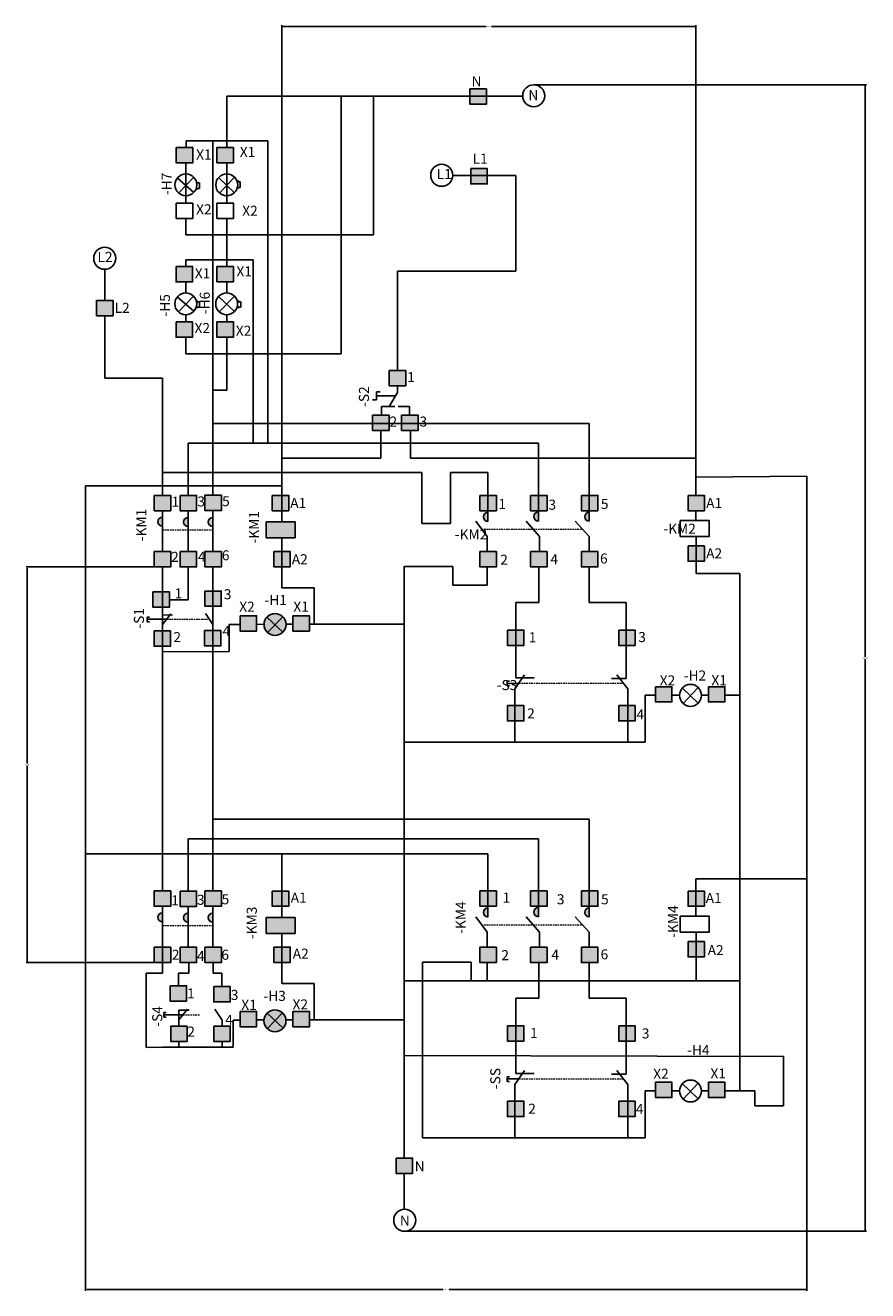
# Model space of a CAD drawing. Units: inches. Extents: x 892 to 1021, y 674 to 867.
import ezdxf

# ---------------------------------------------------------------- set-up
doc = ezdxf.new("R2010")
doc.units = ezdxf.units.IN
doc.header["$MEASUREMENT"] = 0
doc.linetypes.add('DASHED2', pattern=[0.375, 0.25, -0.125])
for name, color, linetype, lineweight in [('A-ANNO-DIMS', 2, 'Continuous', 18), ('E-ANNO-TAGS', 4, 'Continuous', 18), ('E-ANNO-TEXT', 4, 'Continuous', 18), ('E-CTRL-COIL', 7, 'Continuous', 25), ('E-CTRL-CONT', 7, 'Continuous', 25), ('E-CTRL-LAMP', 7, 'Continuous', 25), ('E-CTRL-LINK', 7, 'DASHED2', 18), ('E-CTRL-SWCH', 7, 'Continuous', 25), ('E-CTRL-TERM', 7, 'Continuous', 25), ('E-CTRL-WIRE', 7, 'Continuous', 25), ('E-LAMP-PATT', 1, 'Continuous', 13), ('E-POWR-PORT', 7, 'Continuous', 25), ('E-SYMB-PATT', 7, 'Continuous', 13), ('E-WIRE-NEUT', 4, 'Continuous', 25)]:
    doc.layers.add(name, color=color, linetype=linetype, lineweight=lineweight)
for name, color, linetype, lineweight, true_color in [('E-COIL-PATT', 2, 'Continuous', 13, 0xf1eb1f), ('E-WIRE-L1', 30, 'Continuous', 25, 0xf26722), ('E-WIRE-L2', 219, 'Continuous', 25, 0x642165)]:
    doc.layers.add(name, color=color, linetype=linetype, lineweight=lineweight, true_color=true_color)
doc.styles.get("Standard").update_dxf_attribs({"font": 'arial.ttf'})
doc.dimstyles.get("Standard").update_dxf_attribs({"dimtxt": 0.18, "dimasz": 0.18, "dimexe": 0.18, "dimexo": 0.0625, "dimgap": 0.09, "dimtad": 0, "dimtih": 1, "dimtoh": 1, "dimdec": 4, "dimzin": 0, "dimdsep": 46, "dimtxsty": 'Standard', "dimcen": 0.09, "dimadec": 0, "dimazin": 0, "dimtfac": 1, "dimtdec": 4, "dimtofl": 0, "dimtmove": 0, "dimatfit": 3, "dimfxl": 1, "dimtolj": 1, "dimtzin": 0, "dimarcsym": 0})

# ---------------------------------------------------------------- blocks, each defined once
blk = doc.blocks.new('KM-3POLE-CLOSED')
for p, q in [((1.25, 8.6), (1.25, 2.34)), ((5.18, 8.59), (5.18, 2.34)), ((8.95, 8.62), (8.95, 2.34))]:
    blk.add_line(p, q)
for points in [[(0, 10.95), (2.52, 10.95), (2.52, 8.6), (0, 8.6)], [(3.96, 10.93), (6.48, 10.93), (6.48, 8.59), (3.96, 8.59)], [(7.74, 10.96), (10.26, 10.96), (10.26, 8.62), (7.74, 8.62)], [(0, 2.34), (2.52, 2.34), (2.52, 0), (0, 0)], [(3.96, 2.34), (6.48, 2.34), (6.48, 0), (3.96, 0)], [(7.74, 2.34), (10.26, 2.34), (10.26, 0), (7.74, 0)]]:
    blk.add_lwpolyline(points, close=True)
for centre in [(1.25, 6.92), (5.18, 6.87), (8.95, 6.87)]:
    blk.add_arc(centre, 0.695, 90, 270)
blk = doc.blocks.new('KM-3POLE-OPEN')
for p, q in [((1.87, 10.95), (1.87, 6.96)), ((9.59, 10.95), (9.59, 7.01)), ((17.36, 10.95), (17.36, 6.98)), ((1.73, 4.63), (0, 7)), ((9.77, 4.63), (7.7, 7)), ((15.23, 7), (17.36, 4.63)), ((1.73, 2.34), (1.73, 4.63)), ((9.77, 2.34), (9.77, 4.63)), ((17.36, 4.63), (17.37, 2.34))]:
    blk.add_line(p, q)
for points in [[(0.65, 10.95), (3.17, 10.95), (3.17, 8.6), (0.65, 8.6)], [(8.39, 10.95), (10.91, 10.95), (10.91, 8.6), (8.39, 8.6)], [(16.16, 10.95), (18.68, 10.95), (18.68, 8.6), (16.16, 8.6)], [(0.65, 2.34), (3.17, 2.34), (3.17, 0), (0.65, 0)], [(8.39, 2.34), (10.91, 2.34), (10.91, 0), (8.39, 0)], [(16.16, 2.34), (18.68, 2.34), (18.68, 0), (16.16, 0)]]:
    blk.add_lwpolyline(points, close=True)
for centre in [(1.87, 7.66), (9.59, 7.71), (17.36, 7.67)]:
    blk.add_arc(centre, 0.695, 90, 270)
blk = doc.blocks.new('PB-LINKED-PAIR')
for p, q in [((1.31, 13.88), (1.31, 6.6)), ((18.2, 13.88), (18.21, 6.5)), ((0, 5.74), (0, 6.09)), ((0, 6.09), (0.36, 6.09)), ((1.14, 4.89), (2.64, 7.04)), ((1.31, 6.6), (4.09, 6.6)), ((18.21, 6.5), (15.96, 6.5)), ((18.45, 4.89), (16.77, 7.04)), ((1.73, 5.74), (0, 5.74)), ((0, 5.38), (0, 5.74)), ((0.36, 5.38), (0, 5.38)), ((1.14, 0), (1.14, 4.89)), ((18.45, 0), (18.45, 4.89))]:
    blk.add_line(p, q)
for points in [[(0.02, 13.88), (2.55, 13.88), (2.55, 11.54), (0.02, 11.54)], [(17.04, 13.88), (19.56, 13.88), (19.56, 11.54), (17.04, 11.54)], [(0.02, 2.34), (2.55, 2.34), (2.55, 0), (0.02, 0)], [(17.04, 2.34), (19.56, 2.34), (19.56, 0), (17.04, 0)]]:
    blk.add_lwpolyline(points, close=True)
blk = doc.blocks.new('KM-COIL')
for p, q in [((2.4, 7.73), (2.4, 6.11)), ((2.42, 3.79), (2.43, 2.34))]:
    blk.add_line(p, q)
for points in [[(1.19, 10.07), (3.71, 10.07), (3.71, 7.73), (1.19, 7.73)], [(0, 6.21), (4.44, 6.21), (4.44, 3.79), (0, 3.79)], [(1.19, 2.34), (3.71, 2.34), (3.71, 0), (1.19, 0)]]:
    blk.add_lwpolyline(points, close=True)
blk = doc.blocks.new('PILOT-LAMP-H')
for p, q in [((6.53, 0.48), (4.1, 2.81)), ((4.22, 0.43), (6.54, 2.87)), ((3.67, 1.71), (2.52, 1.7)), ((8.09, 1.72), (7.03, 1.73))]:
    blk.add_line(p, q)
for points in [[(0, 3.01), (2.52, 3.01), (2.52, 0.67), (0, 0.67)], [(8.09, 3.01), (10.61, 3.01), (10.61, 0.67), (8.09, 0.67)]]:
    blk.add_lwpolyline(points, close=True)
blk.add_circle((5.35, 1.68), 1.68)
blk = doc.blocks.new('PILOT-LAMP-V1')
for p, q in [((1.68, 8.48), (1.68, 6.8)), ((2.91, 3.97), (0.37, 6.17)), ((0.55, 3.87), (2.88, 6.3)), ((1.68, 5.05), (1.68, 5.03)), ((1.68, 3.44), (1.68, 2.34))]:
    blk.add_line(p, q)
for points in [[(0.21, 10.83), (2.73, 10.83), (2.73, 8.48), (0.21, 8.48)], [(0.21, 2.34), (2.73, 2.34), (2.73, 0), (0.21, 0)]]:
    blk.add_lwpolyline(points, close=True)
blk.add_circle((1.68, 5.12), 1.68)
blk = doc.blocks.new('PILOT-LAMP-V2')
for p, q in [((1.68, 8.49), (1.68, 6.8)), ((2.86, 3.92), (0.43, 6.24)), ((0.55, 3.87), (2.88, 6.3)), ((1.68, 3.44), (1.68, 2.34))]:
    blk.add_line(p, q)
for points in [[(0.18, 10.83), (2.7, 10.83), (2.7, 8.49), (0.18, 8.49)], [(0.18, 2.34), (2.7, 2.34), (2.7, 0), (0.18, 0)]]:
    blk.add_lwpolyline(points, close=True)
blk.add_circle((1.68, 5.12), 1.68)
blk = doc.blocks.new('SUPPLY-PORT')
blk.add_circle((1.68, 1.68), 1.68)
blk = doc.blocks.new('SCHEM-TERMINAL')
blk.add_lwpolyline([(0, 2.34), (2.52, 2.34), (2.52, 0), (0, 0)], close=True)
blk = doc.blocks.new('*D10')
at = {"layer": 'A-ANNO-DIMS', "color": 0, "lineweight": -2, "transparency": 16777216}
for p, q in [((901.18, 740.67), (901.18, 673.92)), ((1011.49, 736.87), (1011.49, 673.92)), ((901.36, 674.1), (955.88, 674.1)), ((1011.31, 674.1), (956.79, 674.1))]:
    blk.add_line(p, q, dxfattribs=at)
at = {"layer": 'A-ANNO-DIMS', "color": 0, "transparency": 16777216}
for points in [[(901.36, 674.13), (901.36, 674.07), (901.18, 674.1)], [(1011.31, 674.13), (1011.31, 674.07), (1011.49, 674.1)]]:
    blk.add_solid(points, dxfattribs=at)
at = {"layer": 'Defpoints', "color": 0, "transparency": 16777216}
for p in [(901.18, 740.73), (1011.49, 736.93), (1011.49, 674.1)]:
    blk.add_point(p, dxfattribs=at)
at = {"layer": 'A-ANNO-DIMS', "color": 0, "transparency": 16777216, "insert": (956.33, 674.1), "char_height": 0.18, "attachment_point": 5}
blk.add_mtext('\\A1;110.32', dxfattribs=at)
blk = doc.blocks.new('*D11')
at = {"layer": 'A-ANNO-DIMS', "color": 0, "lineweight": -2, "transparency": 16777216}
for p, q in [((969.78, 858.37), (1020.59, 858.37)), ((1020.41, 858.19), (1020.41, 770.88)), ((1020.41, 683.2), (1020.41, 770.51)), ((950.04, 683.02), (1020.59, 683.02))]:
    blk.add_line(p, q, dxfattribs=at)
at = {"layer": 'A-ANNO-DIMS', "color": 0, "transparency": 16777216}
for points in [[(1020.38, 858.19), (1020.44, 858.19), (1020.41, 858.37)], [(1020.38, 683.2), (1020.44, 683.2), (1020.41, 683.02)]]:
    blk.add_solid(points, dxfattribs=at)
at = {"layer": 'Defpoints', "color": 0, "transparency": 16777216}
for p in [(969.71, 858.37), (1020.41, 858.37), (949.98, 683.02)]:
    blk.add_point(p, dxfattribs=at)
at = {"layer": 'A-ANNO-DIMS', "color": 0, "transparency": 16777216, "insert": (1020.41, 770.7), "char_height": 0.18, "attachment_point": 5}
blk.add_mtext('\\A1;175.36', dxfattribs=at)
blk = doc.blocks.new('*D12')
at = {"layer": 'A-ANNO-DIMS', "color": 0, "lineweight": -2, "transparency": 16777216}
for p, q in [((911.61, 784.62), (892.08, 784.62)), ((892.26, 784.44), (892.26, 754.55)), ((892.26, 724.29), (892.26, 754.19)), ((911.61, 724.11), (892.08, 724.11))]:
    blk.add_line(p, q, dxfattribs=at)
at = {"layer": 'A-ANNO-DIMS', "color": 0, "transparency": 16777216}
for points in [[(892.23, 784.44), (892.29, 784.44), (892.26, 784.62)], [(892.23, 724.29), (892.29, 724.29), (892.26, 724.11)]]:
    blk.add_solid(points, dxfattribs=at)
at = {"layer": 'Defpoints', "color": 0, "transparency": 16777216}
for p in [(911.68, 784.62), (892.26, 724.11), (911.68, 724.11)]:
    blk.add_point(p, dxfattribs=at)
at = {"layer": 'A-ANNO-DIMS', "color": 0, "transparency": 16777216, "insert": (892.26, 754.37), "char_height": 0.18, "attachment_point": 5}
blk.add_mtext('\\A1;60.51', dxfattribs=at)
blk = doc.blocks.new('*D13')
at = {"layer": 'A-ANNO-DIMS', "color": 0, "lineweight": -2, "transparency": 16777216}
for p, q in [((931.18, 801.3), (931.18, 867.47)), ((931.36, 867.29), (962.45, 867.29)), ((994.33, 867.29), (963.24, 867.29)), ((994.51, 801.3), (994.51, 867.47))]:
    blk.add_line(p, q, dxfattribs=at)
at = {"layer": 'A-ANNO-DIMS', "color": 0, "transparency": 16777216}
for points in [[(931.36, 867.32), (931.36, 867.26), (931.18, 867.29)], [(994.33, 867.32), (994.33, 867.26), (994.51, 867.29)]]:
    blk.add_solid(points, dxfattribs=at)
at = {"layer": 'Defpoints', "color": 0, "transparency": 16777216}
for p in [(994.51, 867.29), (931.18, 801.24), (994.51, 801.24)]:
    blk.add_point(p, dxfattribs=at)
at = {"layer": 'A-ANNO-DIMS', "color": 0, "transparency": 16777216, "insert": (962.85, 867.29), "char_height": 0.18, "attachment_point": 5}
blk.add_mtext('\\A1;63.33', dxfattribs=at)

msp = doc.modelspace()

# ---------------------------------------------------------------- hatches: boundary and pattern name
at = {"layer": 'E-COIL-PATT'}
h = msp.add_hatch(color=256, dxfattribs=at)
h.dxf.hatch_style = 1
h.paths.add_polyline_path([(928.785, 791.504), (928.785, 789.085), (933.223, 789.085), (933.223, 791.504)])
h = msp.add_hatch(color=256, dxfattribs=at)
h.dxf.hatch_style = 1
h.paths.add_polyline_path([(928.785, 730.993), (928.785, 728.574), (933.223, 728.574), (933.223, 730.993)])
at = {"layer": 'E-LAMP-PATT'}
h = msp.add_hatch(color=256, dxfattribs=at)
h.dxf.hatch_style = 1
h.paths.add_polyline_path([(931.829, 775.823, 0.198195), (931.34, 777.01), (930.143, 775.754), (931.325, 774.622, 0.201366)])
h.paths.add_polyline_path([(931.34, 777.01, 0.4306649), (928.895, 776.948), (930.143, 775.754)])
h.paths.add_polyline_path([(930.143, 775.754), (928.895, 776.948, 0.185153), (928.464, 775.823, 0.2119833), (929.018, 774.575)])
h.paths.add_polyline_path([(930.143, 775.754), (929.018, 774.575, 0.3968623), (931.325, 774.622)])
h.paths.add_polyline_path([(928.943, 716.392), (930.143, 715.243), (931.276, 716.431, 0.4028064)])
h.paths.add_polyline_path([(928.943, 716.392, 0.1995574), (928.447, 715.199, 0.2017164), (928.953, 713.996), (930.143, 715.243)])
h.paths.add_polyline_path([(930.143, 715.243), (928.953, 713.996, 0.424603), (931.374, 714.065)])
h.paths.add_polyline_path([(931.276, 716.431), (930.143, 715.243), (931.374, 714.065, 0.1869519), (931.813, 715.199, 0.2084476)])
at = {"layer": 'E-SYMB-PATT'}
h = msp.add_hatch(color=256, dxfattribs=at)
h.dxf.hatch_style = 1
h.paths.add_polyline_path([(923.773, 822.095), (921.252, 822.095), (921.252, 819.752), (923.773, 819.752)])
h.paths.add_polyline_path([(917.548, 822.095), (915.027, 822.095), (915.027, 819.752), (917.548, 819.752)])
h.paths.add_polyline_path([(917.548, 830.577), (915.027, 830.577), (915.027, 828.234), (917.548, 828.234)])
h.paths.add_polyline_path([(923.773, 830.584), (921.252, 830.584), (921.252, 828.241), (923.773, 828.241)])
h.paths.add_polyline_path([(923.789, 848.777), (921.268, 848.777), (921.268, 846.434), (923.789, 846.434)])
h.paths.add_polyline_path([(917.563, 848.771), (915.042, 848.771), (915.042, 846.428), (917.563, 846.428)])
h.paths.add_polyline_path([(962.466, 857.738), (959.945, 857.738), (959.945, 855.395), (962.466, 855.395)])
h.paths.add_polyline_path([(962.599, 844.476), (960.078, 844.476), (960.078, 843.205), (962.599, 843.205)])
h.paths.add_polyline_path([(962.599, 845.549), (960.078, 845.549), (960.078, 844.476), (962.599, 844.476)])
h.paths.add_polyline_path([(912.924, 731.728, 1), (912.924, 730.337)])
h.paths.add_polyline_path([(914.197, 735.061), (911.676, 735.061), (911.676, 732.718), (914.197, 732.718)])
h.paths.add_polyline_path([(918.157, 735.046), (915.636, 735.046), (915.636, 732.703), (918.157, 732.703)])
h.paths.add_polyline_path([(921.932, 735.077), (919.411, 735.077), (919.411, 732.734), (921.932, 732.734)])
h.paths.add_polyline_path([(920.631, 731.681, 1), (920.631, 730.291)])
h.paths.add_polyline_path([(916.855, 731.681, 1), (916.855, 730.291)])
h.paths.add_polyline_path([(932.249, 735.061), (931.181, 735.061), (931.181, 732.718), (932.249, 732.718)])
h.paths.add_polyline_path([(931.181, 735.061), (929.728, 735.061), (929.728, 732.718), (931.181, 732.718)])
h.paths.add_polyline_path([(962.702, 792.98, 1), (962.702, 791.589)])
h.paths.add_polyline_path([(970.432, 793.031, 1), (970.432, 791.64)])
h.paths.add_polyline_path([(978.2, 792.994, 1), (978.2, 791.603)])
h.paths.add_polyline_path([(947.594, 806.576), (945.073, 806.576), (945.073, 805.51), (947.594, 805.51)])
h.paths.add_polyline_path([(947.594, 807.853), (945.073, 807.853), (945.073, 806.576), (947.594, 806.576)])
h.paths.add_polyline_path([(952.033, 807.853), (949.512, 807.853), (949.512, 806.576), (952.033, 806.576)])
h.paths.add_polyline_path([(952.033, 806.576), (949.512, 806.576), (949.512, 805.51), (952.033, 805.51)])
h.paths.add_polyline_path([(950.127, 814.681), (947.606, 814.681), (947.606, 812.338), (950.127, 812.338)])
h.paths.add_polyline_path([(998.941, 705.799), (996.421, 705.799), (996.421, 703.455), (998.941, 703.455)])
h.paths.add_polyline_path([(990.855, 705.799), (988.334, 705.799), (988.334, 703.455), (990.855, 703.455)])
h = msp.add_hatch(color=256, dxfattribs=at)
h.dxf.hatch_style = 1
h.paths.add_polyline_path([(905.372, 825.387), (902.852, 825.387), (902.852, 823.044), (905.372, 823.044)])
h = msp.add_hatch(color=256, dxfattribs=at)
h.dxf.hatch_style = 1
h.paths.add_polyline_path([(916.705, 714.385), (914.184, 714.385), (914.184, 712.042), (916.705, 712.042)])
h.paths.add_polyline_path([(923.291, 714.392), (920.77, 714.392), (920.77, 712.049), (923.291, 712.049)])
h.paths.add_polyline_path([(927.318, 716.641), (924.797, 716.641), (924.797, 714.298), (927.318, 714.298)])
h.paths.add_polyline_path([(923.294, 720.432), (920.773, 720.432), (920.773, 718.089), (923.294, 718.089)])
h.paths.add_polyline_path([(916.618, 720.563), (914.097, 720.563), (914.097, 718.22), (916.618, 718.22)])
h.paths.add_polyline_path([(918.157, 726.457), (915.636, 726.457), (915.636, 724.114), (918.157, 724.114)])
h.paths.add_polyline_path([(914.197, 726.457), (911.676, 726.457), (911.676, 724.114), (914.197, 724.114)])
h.paths.add_polyline_path([(921.932, 726.457), (919.411, 726.457), (919.411, 724.114), (921.932, 724.114)])
h.paths.add_polyline_path([(931.181, 726.475), (929.962, 726.475), (929.962, 724.132), (931.181, 724.132)])
h.paths.add_polyline_path([(932.483, 726.475), (931.181, 726.475), (931.181, 724.132), (932.483, 724.132)])
h.paths.add_polyline_path([(935.404, 716.641), (932.883, 716.641), (932.883, 714.298), (935.404, 714.298)])
h.paths.add_polyline_path([(984.114, 702.907), (982.697, 702.907), (982.697, 700.564), (984.114, 700.564)])
h.paths.add_polyline_path([(985.218, 702.907), (984.114, 702.907), (984.114, 700.564), (985.218, 700.564)])
h.paths.add_polyline_path([(966.805, 702.907), (965.686, 702.907), (965.686, 700.564), (966.805, 700.564)])
h.paths.add_polyline_path([(968.207, 702.907), (966.805, 702.907), (966.805, 700.564), (968.207, 700.564)])
h.paths.add_polyline_path([(966.969, 714.444), (965.686, 714.444), (965.686, 712.101), (966.969, 712.101)])
h.paths.add_polyline_path([(968.207, 714.444), (966.969, 714.444), (966.969, 712.101), (968.207, 712.101)])
h.paths.add_polyline_path([(985.218, 714.444), (983.862, 714.444), (983.864, 712.101), (985.218, 712.101)])
h.paths.add_polyline_path([(983.862, 714.444), (982.697, 714.444), (982.697, 712.101), (983.864, 712.101)])
h.paths.add_polyline_path([(979.516, 726.457), (976.996, 726.457), (976.996, 724.114), (979.516, 724.114)])
h.paths.add_polyline_path([(971.748, 726.457), (969.228, 726.457), (969.228, 724.114), (971.748, 724.114)])
h.paths.add_polyline_path([(964.004, 726.457), (961.483, 726.457), (961.483, 724.114), (964.004, 724.114)])
h.paths.add_polyline_path([(964.004, 735.061), (962.702, 735.061), (962.702, 732.718), (964.004, 732.718)])
h.paths.add_polyline_path([(962.702, 735.061), (961.483, 735.061), (961.483, 732.718), (962.702, 732.718)])
h.paths.add_polyline_path([(970.432, 735.061), (969.228, 735.061), (969.228, 732.718), (970.432, 732.718)])
h.paths.add_polyline_path([(971.748, 735.061), (970.432, 735.061), (970.432, 732.718), (971.748, 732.718)])
h.paths.add_polyline_path([(978.2, 735.061), (976.996, 735.061), (976.996, 732.718), (978.2, 732.718)])
h.paths.add_polyline_path([(979.516, 735.061), (978.2, 735.061), (978.2, 732.718), (979.516, 732.718)])
h.paths.add_polyline_path([(978.2, 732.483, 1), (978.2, 731.092)])
h.paths.add_polyline_path([(970.432, 732.52, 1), (970.432, 731.129)])
h.paths.add_polyline_path([(962.702, 732.469, 1), (962.702, 731.079)])
h.paths.add_polyline_path([(994.511, 735.061), (993.306, 735.061), (993.306, 732.718), (994.511, 732.718)])
h.paths.add_polyline_path([(995.827, 735.061), (994.511, 735.061), (994.511, 732.718), (995.827, 732.718)])
h.paths.add_polyline_path([(995.827, 727.329), (994.542, 727.329), (994.542, 724.986), (995.827, 724.986)])
h.paths.add_polyline_path([(994.542, 727.329), (993.306, 727.329), (993.306, 724.986), (994.542, 724.986)])
h.paths.add_polyline_path([(998.941, 766.309), (996.421, 766.309), (996.421, 763.966), (998.941, 763.966)])
h.paths.add_polyline_path([(990.855, 766.309), (988.334, 766.309), (988.334, 763.966), (990.855, 763.966)])
h.paths.add_polyline_path([(985.218, 763.418), (984.114, 763.418), (984.114, 761.075), (985.218, 761.075)])
h.paths.add_polyline_path([(984.114, 763.418), (982.697, 763.418), (982.697, 761.075), (984.114, 761.075)])
h.paths.add_polyline_path([(968.207, 763.418), (966.805, 763.418), (966.805, 761.075), (968.207, 761.075)])
h.paths.add_polyline_path([(966.805, 763.418), (965.686, 763.418), (965.686, 761.075), (966.805, 761.075)])
h.paths.add_polyline_path([(966.969, 774.955), (965.686, 774.955), (965.686, 772.612), (966.969, 772.612)])
h.paths.add_polyline_path([(968.207, 774.955), (966.969, 774.955), (966.969, 772.612), (968.207, 772.612)])
h.paths.add_polyline_path([(983.862, 774.955), (982.697, 774.955), (982.697, 772.612), (983.864, 772.612)])
h.paths.add_polyline_path([(985.218, 774.955), (983.862, 774.955), (983.864, 772.612), (985.218, 772.612)])
h.paths.add_polyline_path([(994.542, 787.84), (993.306, 787.84), (993.306, 785.497), (994.542, 785.497)])
h.paths.add_polyline_path([(995.827, 787.84), (994.542, 787.84), (994.542, 785.497), (995.827, 785.497)])
h.paths.add_polyline_path([(995.827, 795.571), (993.306, 795.571), (993.306, 793.228), (995.827, 793.228)])
h.paths.add_polyline_path([(979.516, 795.571), (978.2, 795.571), (978.2, 793.228), (979.516, 793.228)])
h.paths.add_polyline_path([(978.2, 795.571), (976.996, 795.571), (976.996, 793.228), (978.2, 793.228)])
h.paths.add_polyline_path([(971.748, 795.571), (970.432, 795.571), (970.432, 793.228), (971.748, 793.228)])
h.paths.add_polyline_path([(970.432, 795.571), (969.228, 795.571), (969.228, 793.228), (970.432, 793.228)])
h.paths.add_polyline_path([(964.004, 795.571), (962.702, 795.571), (962.702, 793.228), (964.004, 793.228)])
h.paths.add_polyline_path([(962.702, 795.571), (961.483, 795.571), (961.483, 793.228), (962.702, 793.228)])
h.paths.add_polyline_path([(964.004, 786.968), (961.483, 786.968), (961.483, 784.625), (964.004, 784.625)])
h.paths.add_polyline_path([(971.748, 786.968), (969.228, 786.968), (969.228, 784.625), (971.748, 784.625)])
h.paths.add_polyline_path([(979.516, 786.968), (976.996, 786.968), (976.996, 784.625), (979.516, 784.625)])
h.paths.add_polyline_path([(927.318, 777.152), (924.797, 777.152), (924.797, 774.809), (927.318, 774.809)])
h.paths.add_polyline_path([(935.404, 777.152), (932.883, 777.152), (932.883, 774.809), (935.404, 774.809)])
h.paths.add_polyline_path([(932.483, 786.986), (931.181, 786.986), (931.181, 784.643), (932.483, 784.643)])
h.paths.add_polyline_path([(931.181, 786.986), (929.962, 786.986), (929.962, 784.643), (931.181, 784.643)])
h.paths.add_polyline_path([(932.249, 795.571), (931.181, 795.571), (931.181, 793.228), (932.249, 793.228)])
h.paths.add_polyline_path([(931.181, 795.571), (929.728, 795.571), (929.728, 793.228), (931.181, 793.228)])
h.paths.add_polyline_path([(921.932, 795.588), (919.411, 795.588), (919.411, 793.245), (921.932, 793.245)])
h.paths.add_polyline_path([(918.157, 795.557), (915.636, 795.557), (915.636, 793.214), (918.157, 793.214)])
h.paths.add_polyline_path([(914.197, 795.571), (911.676, 795.571), (911.676, 793.228), (914.197, 793.228)])
h.paths.add_polyline_path([(912.924, 792.238, 1), (912.924, 790.848)])
h.paths.add_polyline_path([(916.855, 792.192, 1), (916.855, 790.801)])
h.paths.add_polyline_path([(920.631, 792.192, 1), (920.631, 790.801)])
h.paths.add_polyline_path([(921.932, 786.968), (919.411, 786.968), (919.411, 784.625), (921.932, 784.625)])
h.paths.add_polyline_path([(918.157, 786.968), (915.636, 786.968), (915.636, 784.625), (918.157, 784.625)])
h.paths.add_polyline_path([(914.197, 786.968), (911.676, 786.968), (911.676, 784.625), (914.197, 784.625)])
h.paths.add_polyline_path([(913.996, 780.814), (912.924, 780.814), (912.924, 778.471), (913.996, 778.471)])
h.paths.add_polyline_path([(912.924, 780.814), (911.475, 780.814), (911.475, 778.471), (912.924, 778.471)])
h.paths.add_polyline_path([(912.924, 774.842), (911.652, 774.842), (911.652, 772.499), (912.924, 772.499)])
h.paths.add_polyline_path([(914.173, 774.842), (912.924, 774.842), (912.924, 772.499), (914.173, 772.499)])
h.paths.add_polyline_path([(920.631, 774.9), (919.359, 774.9), (919.359, 772.557), (920.631, 772.557)])
h.paths.add_polyline_path([(921.88, 774.9), (920.631, 774.9), (920.631, 772.557), (921.88, 772.557)])
h.paths.add_polyline_path([(921.932, 780.942), (920.631, 780.942), (920.631, 778.599), (921.932, 778.599)])
h.paths.add_polyline_path([(920.631, 780.942), (919.411, 780.942), (919.411, 778.599), (920.631, 778.599)])
h = msp.add_hatch(color=256, dxfattribs=at)
h.dxf.hatch_style = 1
h.paths.add_polyline_path([(951.193, 694.211), (948.672, 694.211), (948.672, 691.868), (951.193, 691.868)])

# ---------------------------------------------------------------- linework, layer by layer
at = {"layer": 'E-CTRL-COIL'}
for p, q in [((931.181, 795.571), (931.181, 791.403)), ((931.181, 789.085), (931.181, 786.986)), ((931.181, 735.061), (931.181, 730.892)), ((931.181, 728.574), (931.181, 726.475))]:
    msp.add_line(p, q, dxfattribs=at)
for points in [[(928.785, 791.504), (933.223, 791.504), (933.223, 789.085), (928.785, 789.085)], [(928.785, 730.993), (933.223, 730.993), (933.223, 728.574), (928.785, 728.574)]]:
    msp.add_lwpolyline(points, close=True, dxfattribs=at)
at = {"layer": 'E-CTRL-LAMP'}
for p, q in [((918.258, 843.357), (918.258, 843.505)), ((918.258, 843.357), (918.588, 843.357)), ((918.588, 842.513), (918.258, 842.513)), ((918.258, 842.513), (918.258, 842.513)), ((918.258, 842.513), (918.258, 842.355)), ((918.588, 843.357), (918.588, 842.513)), ((924.508, 843.72), (924.508, 843.526)), ((924.508, 843.526), (924.838, 843.526)), ((924.838, 842.682), (924.508, 842.682)), ((924.508, 842.682), (924.508, 842.682)), ((924.508, 842.682), (924.508, 842.524)), ((924.838, 843.526), (924.838, 842.682)), ((918.239, 825.381), (918.239, 825.187)), ((918.239, 825.187), (918.569, 825.187)), ((918.569, 825.187), (918.569, 824.342)), ((924.563, 825.381), (924.563, 825.187)), ((924.563, 825.187), (924.893, 825.187)), ((924.893, 825.187), (924.893, 824.342)), ((918.569, 824.342), (918.239, 824.342)), ((918.239, 824.342), (918.239, 824.342)), ((918.239, 824.342), (918.239, 824.184)), ((924.893, 824.342), (924.563, 824.342)), ((924.563, 824.342), (924.563, 824.342)), ((924.563, 824.342), (924.563, 824.184)), ((931.325, 774.622), (928.895, 776.948)), ((929.018, 774.575), (931.34, 777.01)), ((928.464, 775.846), (927.318, 775.839)), ((932.883, 775.864), (931.829, 775.866)), ((931.374, 714.065), (928.943, 716.392)), ((928.953, 713.996), (931.276, 716.431)), ((928.464, 715.335), (927.318, 715.328)), ((932.883, 715.354), (931.806, 715.356))]:
    msp.add_line(p, q, dxfattribs=at)
for centre in [(930.147, 775.823), (930.13, 715.199)]:
    msp.add_circle(centre, 1.683, dxfattribs=at)
at = {"layer": 'E-CTRL-LINK'}
for p, q in [((912.924, 790.285), (920.631, 790.285)), ((961.741, 790.388), (977.179, 790.388)), ((913.579, 776.646), (920.088, 776.646)), ((983.453, 766.81), (967.395, 766.811)), ((912.924, 729.774), (920.631, 729.774)), ((961.741, 729.877), (977.179, 729.877)), ((916.069, 716.135), (918.688, 716.135)), ((983.453, 706.299), (967.395, 706.3))]:
    msp.add_line(p, q, dxfattribs=at)
at = {"layer": 'E-CTRL-SWCH'}
for p, q in [((945.644, 810.809), (945.644, 811.409)), ((945.644, 811.409), (946.244, 811.409)), ((947.594, 809.165), (948.897, 811.308)), ((948.897, 811.308), (948.897, 812.338)), ((945.644, 810.209), (945.044, 810.209)), ((948.594, 810.809), (945.644, 810.809)), ((945.644, 810.809), (945.644, 810.209)), ((946.424, 807.853), (946.424, 809.165)), ((946.424, 809.165), (948.482, 809.165)), ((950.716, 809.165), (948.985, 809.165)), ((950.716, 807.853), (950.716, 809.165)), ((910.599, 776.592), (910.599, 776.948)), ((910.599, 776.948), (910.955, 776.948)), ((910.599, 776.237), (910.599, 776.592)), ((910.955, 776.237), (910.599, 776.237)), ((913.579, 776.646), (910.641, 776.646)), ((912.924, 775.818), (914.213, 777.445)), ((912.924, 777.307), (914.488, 777.271)), ((920.631, 775.826), (919.524, 777.498)), ((912.924, 774.842), (912.924, 775.818)), ((913.131, 716.135), (913.131, 716.491)), ((913.131, 716.491), (913.487, 716.491)), ((916.069, 716.135), (913.131, 716.135)), ((913.131, 715.779), (913.131, 716.135)), ((915.456, 715.361), (916.745, 716.988)), ((915.456, 716.85), (915.456, 714.385)), ((915.456, 716.85), (917.02, 716.813)), ((922.041, 715.319), (920.934, 716.991)), ((913.487, 715.779), (913.131, 715.779)), ((922.041, 715.319), (922.041, 714.392))]:
    msp.add_line(p, q, dxfattribs=at)
at = {"layer": 'E-CTRL-TERM'}
for points in [[(902.852, 825.387), (905.372, 825.387), (905.372, 823.044), (902.852, 823.044)], [(948.672, 694.211), (951.193, 694.211), (951.193, 691.868), (948.672, 691.868)]]:
    msp.add_lwpolyline(points, close=True, dxfattribs=at)
at = {"layer": 'E-CTRL-WIRE'}
for p, q in [((922.763, 849.78), (916.537, 849.78)), ((916.537, 849.78), (916.537, 848.771)), ((920.631, 849.78), (920.631, 806.576)), ((922.763, 849.78), (929.051, 849.78)), ((922.763, 849.78), (922.768, 848.777)), ((929.051, 849.78), (929.051, 820.743)), ((922.747, 831.586), (916.522, 831.586)), ((916.522, 831.586), (916.522, 830.577)), ((922.747, 831.586), (926.822, 831.586)), ((926.822, 831.586), (926.822, 821.268)), ((926.822, 821.268), (926.822, 803.548)), ((929.051, 820.743), (929.051, 803.548)), ((922.752, 817.205), (922.752, 811.677)), ((922.752, 811.677), (920.631, 811.677)), ((920.631, 806.576), (952.033, 806.576)), ((920.631, 806.576), (920.631, 795.588)), ((946.319, 805.51), (946.319, 801.238)), ((950.841, 805.51), (950.841, 801.238)), ((952.033, 806.576), (973.736, 806.576)), ((973.736, 806.576), (978.2, 806.576)), ((978.2, 806.576), (978.2, 795.571)), ((920.631, 803.548), (916.855, 803.548)), ((916.855, 803.548), (916.855, 795.557)), ((920.631, 803.548), (970.432, 803.548)), ((970.432, 803.548), (970.432, 795.571)), ((946.319, 801.238), (931.181, 801.238)), ((931.181, 801.238), (931.181, 795.571)), ((950.841, 801.238), (984.426, 801.238)), ((984.426, 801.238), (994.511, 801.238)), ((994.511, 801.238), (994.511, 795.571)), ((1011.494, 798.484), (994.511, 798.375)), ((1011.494, 736.935), (1011.494, 798.484)), ((931.181, 797.048), (901.175, 797.048)), ((901.175, 797.048), (901.175, 740.728)), ((912.924, 784.625), (912.924, 775.818)), ((916.855, 784.625), (916.855, 779.583)), ((920.631, 784.625), (920.631, 746.066)), ((957.339, 784.7), (949.897, 784.7)), ((949.897, 784.7), (949.897, 767.061)), ((957.339, 781.822), (957.339, 784.7)), ((962.575, 784.625), (962.575, 781.822)), ((970.491, 779.18), (970.467, 784.625)), ((978.208, 784.625), (978.208, 779.18)), ((962.575, 781.822), (957.339, 781.822)), ((913.996, 779.583), (916.855, 779.583)), ((966.969, 774.955), (966.969, 779.18)), ((966.969, 779.18), (970.491, 779.18)), ((978.208, 779.18), (983.86, 779.18)), ((983.86, 779.18), (983.862, 774.955)), ((912.924, 774.842), (912.924, 738.547)), ((924.797, 775.809), (923.118, 775.809)), ((923.118, 775.809), (923.118, 771.682)), ((923.118, 771.682), (912.924, 771.66)), ((949.897, 767.061), (949.897, 757.82)), ((986.773, 757.82), (986.773, 764.996)), ((988.334, 764.996), (986.773, 764.996)), ((966.805, 761.075), (966.805, 757.82)), ((984.114, 757.82), (984.114, 761.075)), ((949.897, 757.82), (984.114, 757.82)), ((984.114, 757.82), (986.773, 757.82)), ((920.631, 746.066), (952.033, 746.066)), ((920.631, 746.066), (920.631, 735.077)), ((952.033, 746.066), (973.736, 746.066)), ((973.736, 746.066), (978.2, 746.066)), ((978.2, 746.066), (978.2, 735.061)), ((916.855, 743.038), (916.855, 735.046)), ((970.432, 743.038), (916.855, 743.038)), ((970.432, 743.038), (970.432, 735.061)), ((912.924, 740.728), (901.175, 740.728)), ((962.702, 740.728), (912.924, 740.728)), ((931.181, 740.728), (931.181, 735.061)), ((962.702, 735.061), (962.702, 740.728)), ((912.924, 738.547), (912.924, 735.061)), ((994.511, 732.718), (994.511, 736.935)), ((994.511, 736.935), (1011.494, 736.935)), ((912.924, 726.457), (912.924, 722.472)), ((916.957, 722.472), (916.957, 724.114)), ((920.696, 722.469), (920.696, 724.114)), ((960.126, 724.189), (952.684, 724.189)), ((952.684, 724.189), (952.684, 706.55)), ((960.126, 721.312), (960.126, 724.189)), ((962.575, 724.114), (962.575, 721.312)), ((970.491, 718.67), (970.467, 724.114)), ((978.208, 724.114), (978.208, 718.67)), ((912.924, 722.472), (910.421, 722.472)), ((910.421, 722.472), (910.421, 711.144)), ((915.392, 720.563), (915.392, 722.472)), ((915.392, 722.472), (916.957, 722.472)), ((922.007, 722.469), (920.696, 722.469)), ((922.007, 720.432), (922.007, 722.469)), ((960.126, 721.312), (962.575, 721.312)), ((966.969, 714.444), (966.969, 718.67)), ((966.969, 718.67), (970.491, 718.67)), ((978.208, 718.67), (983.86, 718.67)), ((983.86, 718.67), (983.862, 714.444)), ((924.797, 715.298), (923.732, 715.298)), ((923.732, 715.298), (923.732, 711.172)), ((910.421, 711.144), (912.924, 711.149)), ((923.732, 711.173), (912.924, 711.149)), ((915.456, 712.042), (915.456, 711.155)), ((922.041, 712.049), (922.041, 711.169)), ((952.684, 706.55), (952.684, 697.309)), ((986.773, 697.309), (986.773, 704.486)), ((988.334, 704.486), (986.773, 704.486)), ((966.805, 700.564), (966.805, 697.309)), ((984.114, 697.309), (984.114, 700.564)), ((952.684, 697.309), (984.114, 697.309)), ((984.114, 697.309), (986.773, 697.309))]:
    msp.add_line(p, q, dxfattribs=at)
at = {"layer": 'E-WIRE-L1'}
for p, q in [((962.599, 844.476), (957.322, 844.476)), ((966.952, 844.476), (962.599, 844.476)), ((966.952, 829.841), (966.952, 844.476)), ((948.895, 814.681), (948.895, 829.841)), ((948.895, 829.841), (966.952, 829.841))]:
    msp.add_line(p, q, dxfattribs=at)
at = {"layer": 'E-WIRE-L2'}
for p, q in [((904.098, 825.387), (904.098, 830.154)), ((904.098, 813.484), (904.098, 823.044)), ((912.924, 813.484), (904.098, 813.484)), ((912.924, 799.058), (912.924, 813.484)), ((952.608, 799.058), (912.924, 799.058)), ((912.924, 799.058), (912.924, 795.571)), ((952.608, 791.272), (952.608, 799.058)), ((962.702, 799.058), (956.989, 799.058)), ((956.989, 799.058), (956.989, 791.272)), ((962.702, 795.571), (962.702, 799.058)), ((956.989, 791.272), (952.608, 791.272))]:
    msp.add_line(p, q, dxfattribs=at)
at = {"layer": 'E-WIRE-NEUT'}
for p, q in [((922.763, 856.63), (959.945, 856.63)), ((922.763, 856.63), (922.763, 849.78)), ((940.278, 856.63), (940.278, 817.205)), ((945.192, 835.399), (945.19, 856.63)), ((959.945, 856.63), (968.097, 856.63)), ((916.514, 844.746), (916.508, 841.381)), ((922.768, 844.746), (922.768, 841.381)), ((916.514, 835.399), (916.514, 837.945)), ((922.768, 837.945), (922.768, 833.358)), ((922.763, 835.399), (916.514, 835.399)), ((922.763, 835.399), (945.192, 835.399)), ((922.768, 833.358), (922.768, 831.586)), ((922.768, 831.586), (922.765, 830.584)), ((916.498, 817.205), (916.498, 819.752)), ((922.752, 819.752), (922.752, 817.205)), ((922.747, 817.205), (916.498, 817.205)), ((922.752, 817.205), (940.278, 817.205)), ((994.542, 787.84), (994.542, 783.605)), ((931.181, 786.986), (931.181, 781.426)), ((994.542, 783.605), (1001.248, 783.605)), ((1001.248, 783.605), (1001.248, 736.935)), ((931.181, 781.426), (936.134, 781.426)), ((936.134, 781.426), (936.134, 775.86)), ((935.404, 775.86), (949.897, 775.86)), ((949.897, 775.86), (949.897, 696.442)), ((998.941, 765.022), (1001.248, 765.022)), ((1001.248, 736.935), (1001.248, 704.511)), ((931.181, 726.475), (931.181, 720.916)), ((994.542, 727.329), (994.542, 721.312)), ((931.181, 720.916), (936.134, 720.916)), ((936.134, 720.916), (936.134, 715.349)), ((949.897, 721.312), (1001.248, 721.312)), ((935.404, 715.349), (949.897, 715.349)), ((1007.922, 709.741), (949.897, 709.884)), ((1007.922, 702.216), (1007.922, 709.741)), ((998.941, 704.511), (1001.248, 704.511)), ((1001.248, 704.511), (1003.509, 704.511)), ((1003.509, 704.511), (1003.509, 702.216)), ((1003.509, 702.216), (1007.922, 702.216)), ((949.897, 696.442), (949.897, 694.211)), ((949.897, 691.868), (949.897, 689.401)), ((949.897, 689.401), (949.897, 686.381))]:
    msp.add_line(p, q, dxfattribs=at)

# ---------------------------------------------------------------- block references
at = {"layer": 'E-CTRL-COIL'}
for p in [(992.114, 785.497), (992.114, 724.986)]:
    msp.add_blockref('KM-COIL', p, dxfattribs=at)
at = {"layer": 'E-CTRL-CONT'}
for name, p in [('KM-3POLE-CLOSED', (911.676, 784.625)), ('KM-3POLE-OPEN', (960.837, 784.625)), ('KM-3POLE-CLOSED', (911.676, 724.114)), ('KM-3POLE-OPEN', (960.837, 724.114))]:
    msp.add_blockref(name, p, dxfattribs=at)
at = {"layer": 'E-CTRL-LAMP'}
for name, p in [('PILOT-LAMP-V1', (914.831, 837.945)), ('PILOT-LAMP-V2', (921.085, 837.945)), ('PILOT-LAMP-V1', (914.815, 819.751)), ('PILOT-LAMP-V2', (921.069, 819.751)), ('PILOT-LAMP-H', (988.334, 763.298)), ('PILOT-LAMP-H', (988.334, 702.787))]:
    msp.add_blockref(name, p, dxfattribs=at)
at = {"layer": 'E-CTRL-SWCH'}
for p in [(965.661, 761.075), (965.661, 700.564)]:
    msp.add_blockref('PB-LINKED-PAIR', p, dxfattribs=at)
at = {"layer": 'E-CTRL-TERM'}
for p in [(959.945, 855.395), (960.078, 843.205), (947.606, 812.338), (945.073, 805.509), (949.512, 805.509), (929.728, 793.228), (929.962, 784.643), (911.475, 778.471), (919.412, 778.599), (924.797, 774.808), (932.884, 774.808), (911.652, 772.499), (919.359, 772.556), (929.728, 732.717), (929.962, 724.132), (914.097, 718.22), (920.773, 718.088), (924.797, 714.298), (932.884, 714.298), (914.184, 712.042), (920.77, 712.049)]:
    msp.add_blockref('SCHEM-TERMINAL', p, dxfattribs=at)
at = {"layer": 'E-POWR-PORT'}
for p in [(968.031, 855.009), (953.958, 842.853), (902.422, 830.154), (948.294, 683.018)]:
    msp.add_blockref('SUPPLY-PORT', p, dxfattribs=at)

# ---------------------------------------------------------------- texts
at = {"layer": 'E-ANNO-TAGS'}
for s, p in [('-H7', (914.341, 841.499)), ('-H6', (920.172, 823.282)), ('-H5', (914.076, 822.932)), ('-S2', (944.516, 809.103)), ('-KM1', (910.447, 788.564)), ('-KM1', (927.693, 788.224)), ('-S1', (910.1, 775.197)), ('-KM3', (927.355, 727.712)), ('-KM4', (959.32, 728.513)), ('-KM4', (991.779, 727.909)), ('-S4', (912.902, 714.307)), ('-SS', (964.603, 704.75))]:
    msp.add_text(s, height=1.5385, rotation=90, dxfattribs=at).set_placement(p)
for s, p in [('-KM2', (957.642, 788.824)), ('-KM2', (989.546, 789.691)), ('-H1', (928.534, 778.803)), ('-H2', (992.656, 767.246)), ('-S3', (964.05, 765.791)), ('-H3', (928.378, 718.251)), ('-H4', (993.177, 709.96))]:
    msp.add_text(s, height=1.5385, dxfattribs=at).set_placement(p)
at = {"layer": 'E-ANNO-TEXT'}
for s, height, p in [('N', 1.538, (960.201, 858.14)), ('N', 1.538, (968.891, 856.019)), ('X1', 1.5385, (918.077, 846.937)), ('X1', 1.5385, (924.759, 847.334)), ('L1', 1.5385, (960.359, 846.316)), ('L1', 1.5385, (954.868, 843.947)), ('X2', 1.5385, (918.077, 838.554)), ('X2', 1.5385, (925.13, 838.336)), ('L2', 1.5385, (902.989, 831.278)), ('X1', 1.5385, (924.246, 829.062)), ('X1', 1.5385, (917.871, 828.767)), ('L2', 1.5385, (905.612, 823.482)), ('X2', 1.5385, (917.838, 820.396)), ('X2', 1.5385, (924.147, 819.979)), ('1', 1.538, (950.351, 812.893)), ('2', 1.538, (947.654, 806.086)), ('3', 1.538, (952.243, 806.086)), ('1', 1.538, (914.329, 793.845)), ('3', 1.538, (918.269, 793.871)), ('5', 1.538, (922.053, 793.91)), ('A1', 1.5385, (932.467, 793.636)), ('1', 1.538, (964.306, 793.482)), ('3', 1.538, (971.96, 793.374)), ('5', 1.538, (979.975, 793.482)), ('A1', 1.5385, (996.084, 793.627)), ('2', 1.538, (914.252, 785.398)), ('4', 1.538, (918.353, 785.411)), ('6', 1.538, (922.01, 785.634)), ('A2', 1.5385, (932.713, 785.028)), ('2', 1.538, (964.589, 784.961)), ('4', 1.538, (972.258, 785.038)), ('6', 1.538, (979.85, 785.147)), ('A2', 1.5385, (996.084, 785.918)), ('1', 1.538, (914.792, 779.809)), ('3', 1.538, (922.309, 779.678)), ('X2', 1.5385, (924.669, 777.775)), ('X1', 1.5385, (932.943, 777.779)), ('2', 1.538, (914.601, 773.13)), ('4', 1.538, (922.114, 774.041)), ('1', 1.538, (968.947, 773.104)), ('3', 1.538, (985.695, 773.129)), ('X2', 1.5385, (988.973, 766.501)), ('X1', 1.5385, (996.883, 766.532)), ('2', 1.538, (968.708, 761.452)), ('4', 1.538, (985.416, 761.291)), ('1', 1.538, (914.272, 732.864)), ('3', 1.538, (918.209, 732.954)), ('5', 1.538, (921.986, 733.025)), ('A1', 1.5385, (932.546, 733.269)), ('1', 1.538, (964.944, 733.279)), ('3', 1.538, (973.245, 733.022)), ('5', 1.538, (980.002, 733.022)), ('A1', 1.5385, (996.012, 733.223)), ('2', 1.538, (914.362, 724.543)), ('4', 1.538, (918.222, 724.358)), ('6', 1.538, (921.941, 724.539)), ('A2', 1.5385, (932.855, 724.701)), ('2', 1.538, (964.751, 724.471)), ('4', 1.538, (972.409, 724.535)), ('6', 1.538, (979.937, 724.6)), ('A2', 1.5385, (996.314, 725.244)), ('1', 1.538, (916.692, 718.617)), ('3', 1.538, (923.382, 718.395)), ('X1', 1.5385, (924.983, 716.874)), ('X2', 1.5385, (932.824, 716.943)), ('2', 1.538, (916.735, 712.782)), ('4', 1.538, (922.528, 714.578)), ('1', 1.538, (969.152, 712.571)), ('3', 1.538, (986.238, 712.507)), ('X2', 1.5385, (987.985, 706.335)), ('X1', 1.5385, (996.736, 706.379)), ('2', 1.538, (968.865, 700.988)), ('4', 1.538, (985.331, 700.951)), ('N', 1.538, (951.511, 692.157)), ('N', 1.538, (949.244, 683.861))]:
    msp.add_text(s, height=height, dxfattribs=at).set_placement(p)

# ---------------------------------------------------------------- dimensions: what is measured, and where the dimension line sits
at = {"layer": 'A-ANNO-DIMS'}
for base, p1, p2, picture, middle in [((994.511, 867.289), (931.181, 801.238), (994.511, 801.238), '*D13', (962.846, 867.289)), ((1011.494, 674.103), (901.175, 740.728), (1011.494, 736.935), '*D10', (956.335, 674.103))]:
    dim = msp.add_linear_dim(base=base, p1=p1, p2=p2, dimstyle='Standard', override={"dimdec": 2, "dimlfac": 1, "dimrnd": 0, "dimzin": 0, "dimdsep": 46, "dimlunit": 2}, dxfattribs=at)
    dim.commit()
    dim.dimension.update_dxf_attribs({"geometry": picture, "text_midpoint": middle})
for base, p1, p2, picture, middle in [((1020.409, 858.374), (949.977, 683.018), (969.713, 858.374), '*D11', (1020.409, 770.696)), ((892.26, 724.114), (911.676, 784.625), (911.676, 724.114), '*D12', (892.26, 754.369))]:
    dim = msp.add_linear_dim(base=base, p1=p1, p2=p2, angle=90, dimstyle='Standard', override={"dimdec": 2, "dimlfac": 1, "dimrnd": 0, "dimzin": 0, "dimdsep": 46, "dimlunit": 2}, dxfattribs=at)
    dim.commit()
    dim.dimension.update_dxf_attribs({"geometry": picture, "text_midpoint": middle})

doc.saveas('drawing.dxf')
